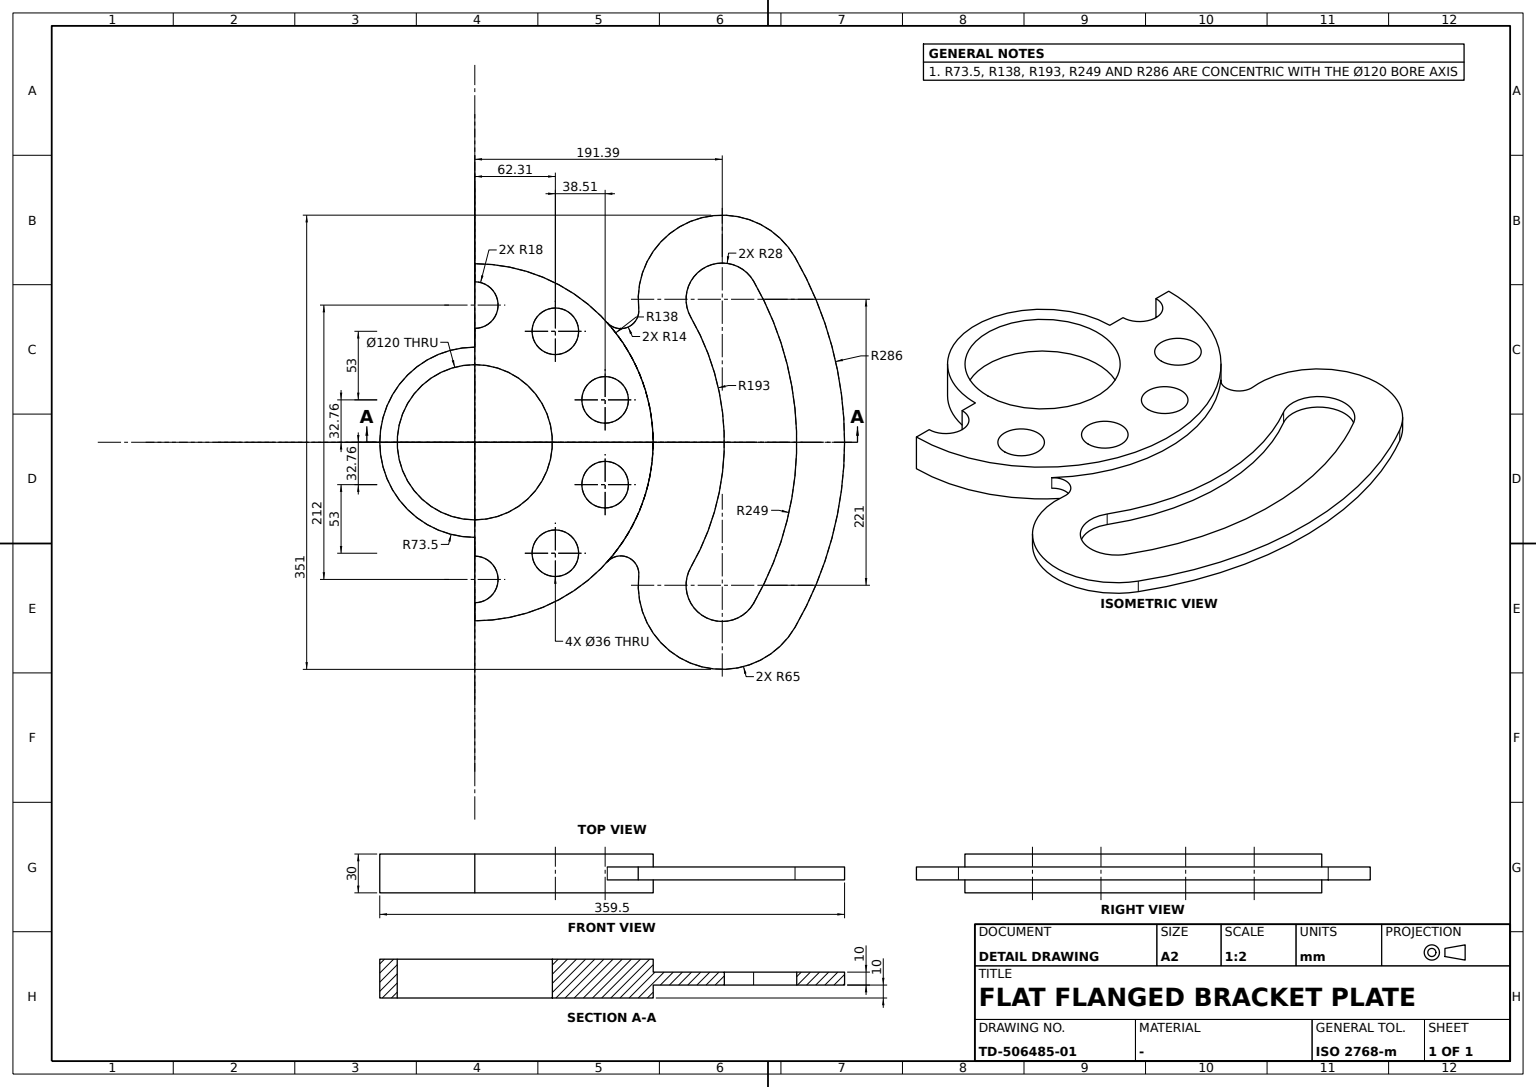
CATIA V5 part; units mm, degrees
sketch "Sketch1" plane through (0, 0, 0) normal (0, 0, 1) x (1, 0, 0)
  circle A0 centre (0, 0) radius 60
  arc A1 (73.5, 0) -> (-73.5, 0) centre (0, 0) ccw construction
  arc A2 (138, 0) -> (92.427, 102.4756) centre (0, 0) ccw
  line L0 (-234.3613, 0) -> (236.032, 0) construction
  point P0 (-234.3613, 0)
  circle A3 centre (0, 0) radius 106 construction
  line L1 (73.5, 0) -> (138, 0)
  point P1 (73.5, 0)
  point P2 (138, 0)
  line L2 (-73.5, 0) -> (-138, 0)
  point P3 (-73.5, 0)
  point P4 (-138, 0)
  point P5 (-138, 0)
  point P6 (138, 0)
  point P7 (-73.5, 0)
  point P8 (73.5, 0)
  point P9 (105.75, 0)
  line L3 (0, 0) -> (-180.5765, 312.7676) construction
  point P10 (-180.5765, 312.7676)
  point P11 (180.5765, 312.7676)
  point P12 (0, 0)
  line L4 (0, 0) -> (180.5765, 312.7676) construction
  circle A4 centre (0, 0) radius 221 construction
  arc A5 (110.5, 191.3916) -> (-110.5, 191.3916) centre (0, 0) ccw construction
  point P13 (-110.5, 191.3916)
  point P14 (110.5, 191.3916)
  arc A6 (143, 247.6833) -> (103.3447, 126.7866) centre (110.5, 191.3916) cw
  arc A7 (-103.3447, 126.7866) -> (-143, 247.6833) centre (-110.5, 191.3916) cw
  arc A8 (-143, 247.6833) -> (143, 247.6833) centre (0, 0) cw
  arc A9 (110.5, 191.3916) -> (-110.5, 191.3916) centre (0, 0) ccw construction
  arc A10 (124.5, 215.6403) -> (96.5, 167.1429) centre (110.5, 191.3916) cw
  arc A11 (-96.5, 167.1429) -> (-124.5, 215.6403) centre (-110.5, 191.3916) cw
  arc A12 (96.5, 167.1429) -> (-96.5, 167.1429) centre (0, 0) ccw
  arc A13 (-124.5, 215.6403) -> (124.5, 215.6403) centre (0, 0) cw
  arc A14 (103.3447, 126.7866) -> (92.427, 102.4756) centre (101.8036, 112.8717) ccw
  arc A15 (-103.3447, 126.7866) -> (-92.427, 102.4756) centre (-101.8036, 112.8717) cw
  point P15 (-92.427, 102.4756)
  arc A16 (-92.427, 102.4756) -> (-138, 0) centre (0, 0) ccw
  arc A17 (-73.5, 0) -> (73.5, 0) centre (0, 0) ccw
  point P16 (0, 73.5)
  dimension "radius A0" = 60
  dimension "radius A1" = 73.5
  dimension "radius A2" = 138
  dimension "radius A3" = 106
  dimension "angle y axis L3" = 30
  dimension "radius A4" = 221
  dimension "radius A7" = 65
  dimension "radius A11" = 28
  dimension "radius A14" = 14
  constraint coincidence P0 x-axis
  constraint coincidence P1 A1
  constraint coincidence P1 L0
  constraint coincidence P2 A2
  constraint coincidence P3 A1
  constraint coincidence P3 L0
  constraint coincidence P4 A2
  constraint coincidence L0 P5
  constraint coincidence L0 P6
  constraint coincidence L0 P7
  constraint coincidence L0 P8
  constraint coincidence P13 A4
  constraint coincidence P13 L3
  constraint coincidence P14 L4
  constraint coincidence A2 P15
  constraint coincidence A2 A16
  constraint coincidence A17 P16
  constraint coincidence P16 A1
  constraint coincidence P16 y-axis
  constraint coincidence P1 P8
  constraint coincidence P2 P6
  constraint coincidence P3 P7
  constraint coincidence P4 P5
  constraint horizontal L0 x-axis
  constraint horizontal L1 x-axis
  constraint horizontal L2 x-axis
  constraint midpoint P9 L1
  constraint symmetry P10 P11 y-axis
  constraint symmetry origin P12 y-axis
  constraint symmetry L3 L4 y-axis
  constraint symmetry A14 A15 y-axis
  constraint tangency A7 A8
  constraint tangency A8 A6
  constraint tangency A12 A11
  constraint tangency A11 A13
  constraint tangency A13 A10
  constraint tangency A10 A12
  constraint tangency A14 A6
  constraint tangency A14 A2
  constraint concentricity A8 origin
  constraint concentricity A12 origin
  constraint concentricity A13 origin
extrude "Pad1" add sketch "Sketch1" along normal mid plane 10
sketch "Sketch2" plane through (0, 0, 0) normal (0, 0, 1) x (1, 0, 0)
  line L0 (-138, 0) -> (-73.5, 0)
  circle A0 centre (0, 0) radius 60
  line L1 (73.5, 0) -> (138, 0)
  arc A1 (-73.5, 0) -> (73.5, 0) centre (0, 0) ccw
  arc A2 (138, 0) -> (-138, 0) centre (0, 0) ccw
extrude "Pad2" add sketch "Sketch2" along normal mid plane 30
sketch "Sketch3" plane through (0, 0, 15) normal (0, 0, 1) x (1, 0, 0)
  circle A0 centre (0, 0) radius 106 construction
  circle A1 centre (106, 0) radius 18
  point P0 (106, 0)
  dimension "radius A0" = 106
  dimension "radius A1" = 18
  constraint coincidence P0 A0
  constraint coincidence P0 x-axis
extrude "Pocket1" cut sketch "Sketch3" against normal blind 30
pattern_circular "CircPattern1" count 6 over 180 about axis through (0, 0, 0) along (0, 0, 1) of "Pocket1"
